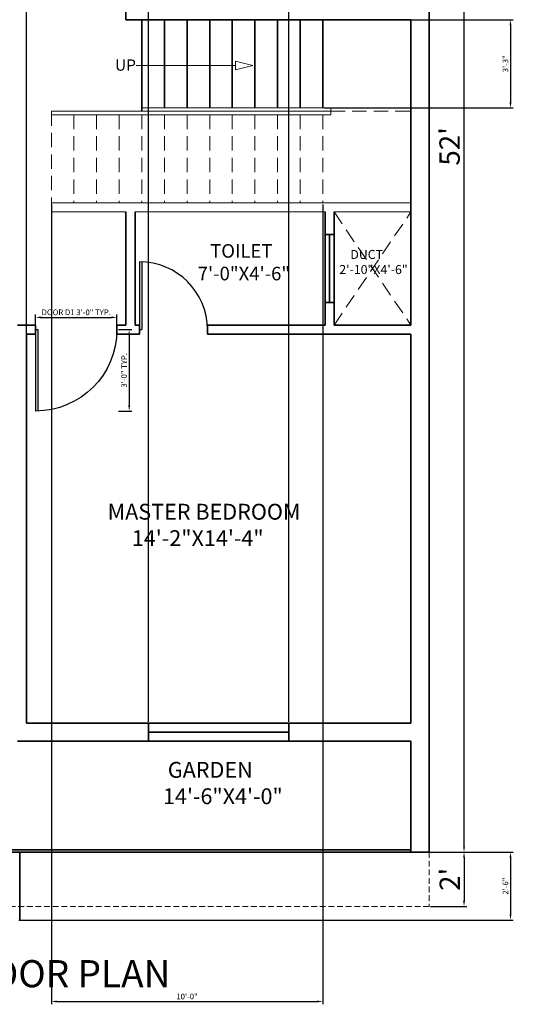
# Model space of a CAD drawing. Units: inches. Extents: x 1566 to 2546, y 1087 to 2705.
# Tile 25 of 27: x 1821 to 2039, y 1974 to 2409. Entities that reach past the tile are written whole.
import ezdxf

# ---------------------------------------------------------------- set-up
doc = ezdxf.new("R2010")
doc.units = ezdxf.units.IN
doc.linetypes.add('DASHED', pattern=[19.05, 12.7, -6.35])
for name, color, linetype, lineweight in [('A-ANNO-DIMS', 2, 'Continuous', 18), ('A-ANNO-TEXT', 7, 'Continuous', 18), ('A-AREA-IDEN', 7, 'Continuous', 18), ('A-DOOR', 4, 'Continuous', 25), ('A-FLOR-OVHD', 8, 'DASHED', 18), ('A-FLOR-STRS', 3, 'Continuous', 18), ('A-WALL', 7, 'Continuous', 35)]:
    doc.layers.add(name, color=color, linetype=linetype, lineweight=lineweight)
doc.styles.get("Standard").update_dxf_attribs({"font": 'arial.ttf'})
doc.dimstyles.new('ISO-25', dxfattribs={"dimtxt": 2.5, "dimasz": 2.5, "dimexe": 1.25, "dimexo": 0.625, "dimtad": 1, "dimtxsty": 'Standard', "dimcen": 2.5, "dimadec": 0, "dimazin": 0, "dimtfac": 1, "dimtmove": 0, "dimatfit": 3, "dimfxl": 1, "dimarcsym": 0})

# ---------------------------------------------------------------- blocks, each defined once
blk = doc.blocks.new('d2')
for p, q in [((3364.08, 1632.29), (3364.08, 1602.29)), ((3365.08, 1632.29), (3365.08, 1602.29)), ((3364.08, 1602.29), (3365.08, 1602.29))]:
    blk.add_line(p, q)
at = {"ltscale": 0.3}
blk.add_arc((3364.08, 1602.29), 30, 0, 90, dxfattribs=at)
blk = doc.blocks.new('d1')
for p, q in [((3297.32, 1596.93), (3297.32, 1632.93)), ((3298.32, 1596.93), (3298.32, 1632.93)), ((3297.32, 1596.93), (3298.32, 1596.93))]:
    blk.add_line(p, q)
at = {"ltscale": 0.3}
blk.add_arc((3297.32, 1596.93), 36, 0, 90, dxfattribs=at)
blk = doc.blocks.new('*D12')
at = {"layer": 'A-ANNO-DIMS', "color": 0, "lineweight": -2, "transparency": 16777216}
for p, q in [((2002.15, 2665.35), (2018.24, 2665.35)), ((2016.99, 2043.85), (2016.99, 2662.85)), ((2002.15, 2041.35), (2018.24, 2041.35))]:
    blk.add_line(p, q, dxfattribs=at)
at = {"layer": 'A-ANNO-DIMS', "color": 0, "transparency": 16777216}
for points in [[(2016.58, 2662.85), (2017.41, 2662.85), (2016.99, 2665.35)], [(2016.58, 2043.85), (2017.41, 2043.85), (2016.99, 2041.35)]]:
    blk.add_solid(points, dxfattribs=at)
at = {"layer": 'Defpoints', "color": 0, "transparency": 16777216}
for p in [(2001.53, 2665.35), (2016.99, 2665.35), (2001.53, 2041.35)]:
    blk.add_point(p, dxfattribs=at)
at = {"layer": 'A-ANNO-DIMS', "color": 0, "transparency": 16777216, "insert": (2011.77, 2353.35), "char_height": 9, "attachment_point": 5, "rotation": 90}
blk.add_mtext("52'", dxfattribs=at)
blk = doc.blocks.new('*D14')
at = {"layer": 'A-ANNO-DIMS', "color": 0, "lineweight": -2, "transparency": 16777216}
for p, q in [((2002.15, 2041.35), (2018.24, 2041.35)), ((2016.99, 2038.85), (2016.99, 2019.85)), ((2002.15, 2017.35), (2018.24, 2017.35))]:
    blk.add_line(p, q, dxfattribs=at)
at = {"layer": 'A-ANNO-DIMS', "color": 0, "transparency": 16777216}
for points in [[(2016.58, 2038.85), (2017.41, 2038.85), (2016.99, 2041.35)], [(2016.58, 2019.85), (2017.41, 2019.85), (2016.99, 2017.35)]]:
    blk.add_solid(points, dxfattribs=at)
at = {"layer": 'Defpoints', "color": 0, "transparency": 16777216}
for p in [(2001.53, 2041.35), (2001.53, 2017.35), (2016.99, 2017.35)]:
    blk.add_point(p, dxfattribs=at)
at = {"layer": 'A-ANNO-DIMS', "color": 0, "transparency": 16777216, "insert": (2011.85, 2029.35), "char_height": 9, "attachment_point": 5, "rotation": 90}
blk.add_mtext("2'", dxfattribs=at)
blk = doc.blocks.new('*D35')
at = {"layer": 'A-ANNO-DIMS', "color": 0, "lineweight": -2, "transparency": 16777216}
for p, q in [((1827.53, 2272.97), (1827.53, 2279)), ((1830.03, 2277.75), (1861.03, 2277.75)), ((1863.53, 2272.97), (1863.53, 2279))]:
    blk.add_line(p, q, dxfattribs=at)
at = {"layer": 'A-ANNO-DIMS', "color": 0, "transparency": 16777216}
for points in [[(1830.03, 2278.16), (1830.03, 2277.33), (1827.53, 2277.75)], [(1861.03, 2278.16), (1861.03, 2277.33), (1863.53, 2277.75)]]:
    blk.add_solid(points, dxfattribs=at)
at = {"layer": 'Defpoints', "color": 0, "transparency": 16777216}
for p in [(1863.53, 2277.75), (1827.53, 2272.35), (1863.53, 2272.35)]:
    blk.add_point(p, dxfattribs=at)
at = {"layer": 'A-ANNO-DIMS', "color": 0, "transparency": 16777216, "insert": (1845.53, 2279.67), "char_height": 2.5, "attachment_point": 5}
blk.add_mtext('DOOR D1 3\'-0" TYP.', dxfattribs=at)
blk = doc.blocks.new('*D36')
at = {"layer": 'A-ANNO-DIMS', "color": 0, "lineweight": -2, "transparency": 16777216}
for p, q in [((1864.15, 2272.35), (1870.18, 2272.35)), ((1868.93, 2269.85), (1868.93, 2238.85)), ((1864.15, 2236.35), (1870.18, 2236.35))]:
    blk.add_line(p, q, dxfattribs=at)
at = {"layer": 'A-ANNO-DIMS', "color": 0, "transparency": 16777216}
for points in [[(1868.51, 2269.85), (1869.35, 2269.85), (1868.93, 2272.35)], [(1868.51, 2238.85), (1869.35, 2238.85), (1868.93, 2236.35)]]:
    blk.add_solid(points, dxfattribs=at)
at = {"layer": 'Defpoints', "color": 0, "transparency": 16777216}
for p in [(1863.53, 2272.35), (1863.53, 2236.35), (1868.93, 2236.35)]:
    blk.add_point(p, dxfattribs=at)
at = {"layer": 'A-ANNO-DIMS', "color": 0, "transparency": 16777216, "insert": (1867.03, 2254.35), "char_height": 2.5, "attachment_point": 5, "rotation": 90}
blk.add_mtext('3\'-0" TYP.', dxfattribs=at)
blk = doc.blocks.new('*D81')
at = {"layer": 'A-ANNO-DIMS', "color": 0, "lineweight": -2, "transparency": 16777216}
for p, q in [((1823.53, 2098.97), (1823.53, 2702.6)), ((1826.03, 2701.35), (1875.03, 2701.35)), ((1877.53, 2098.97), (1877.53, 2702.6))]:
    blk.add_line(p, q, dxfattribs=at)
at = {"layer": 'A-ANNO-DIMS', "color": 0, "transparency": 16777216}
for points in [[(1826.03, 2701.76), (1826.03, 2700.93), (1823.53, 2701.35)], [(1875.03, 2701.76), (1875.03, 2700.93), (1877.53, 2701.35)]]:
    blk.add_solid(points, dxfattribs=at)
at = {"layer": 'Defpoints', "color": 0, "transparency": 16777216}
for p in [(1877.53, 2701.35), (1823.53, 2098.35), (1877.53, 2098.35)]:
    blk.add_point(p, dxfattribs=at)
at = {"layer": 'A-ANNO-DIMS', "color": 0, "transparency": 16777216, "insert": (1850.53, 2703.25), "char_height": 2.5, "attachment_point": 5}
blk.add_mtext('4\'-6"', dxfattribs=at)
blk = doc.blocks.new('*D82')
at = {"layer": 'A-ANNO-DIMS', "color": 0, "lineweight": -2, "transparency": 16777216}
for p, q in [((1877.53, 2098.97), (1877.53, 2702.6)), ((1880.03, 2701.35), (1937.03, 2701.35)), ((1939.53, 2098.97), (1939.53, 2702.6))]:
    blk.add_line(p, q, dxfattribs=at)
at = {"layer": 'A-ANNO-DIMS', "color": 0, "transparency": 16777216}
for points in [[(1880.03, 2701.76), (1880.03, 2700.93), (1877.53, 2701.35)], [(1937.03, 2701.76), (1937.03, 2700.93), (1939.53, 2701.35)]]:
    blk.add_solid(points, dxfattribs=at)
at = {"layer": 'Defpoints', "color": 0, "transparency": 16777216}
for p in [(1939.53, 2701.35), (1877.53, 2098.35), (1939.53, 2098.35)]:
    blk.add_point(p, dxfattribs=at)
at = {"layer": 'A-ANNO-DIMS', "color": 0, "transparency": 16777216, "insert": (1908.53, 2703.25), "char_height": 2.5, "attachment_point": 5}
blk.add_mtext('5\'-2"', dxfattribs=at)
blk = doc.blocks.new('*D84')
at = {"layer": 'A-ANNO-DIMS', "color": 0, "lineweight": -2, "transparency": 16777216}
for p, q in [((1955.15, 2409.35), (2038.78, 2409.35)), ((2037.53, 2406.85), (2037.53, 2372.85)), ((1955.15, 2370.35), (2038.78, 2370.35))]:
    blk.add_line(p, q, dxfattribs=at)
at = {"layer": 'A-ANNO-DIMS', "color": 0, "transparency": 16777216}
for points in [[(2037.11, 2406.85), (2037.95, 2406.85), (2037.53, 2409.35)], [(2037.11, 2372.85), (2037.95, 2372.85), (2037.53, 2370.35)]]:
    blk.add_solid(points, dxfattribs=at)
at = {"layer": 'Defpoints', "color": 0, "transparency": 16777216}
for p in [(1954.53, 2409.35), (1954.53, 2370.35), (2037.53, 2370.35)]:
    blk.add_point(p, dxfattribs=at)
at = {"layer": 'A-ANNO-DIMS', "color": 0, "transparency": 16777216, "insert": (2035.63, 2389.85), "char_height": 2.5, "attachment_point": 5, "rotation": 90}
blk.add_mtext('3\'-3"', dxfattribs=at)
blk = doc.blocks.new('*D85')
at = {"layer": 'A-ANNO-DIMS', "color": 0, "lineweight": -2, "transparency": 16777216}
for p, q in [((1834.53, 2327.72), (1834.53, 1974.1)), ((1954.53, 2327.72), (1954.53, 1974.1)), ((1837.03, 1975.35), (1952.03, 1975.35))]:
    blk.add_line(p, q, dxfattribs=at)
at = {"layer": 'A-ANNO-DIMS', "color": 0, "transparency": 16777216}
for points in [[(1837.03, 1975.76), (1837.03, 1974.93), (1834.53, 1975.35)], [(1952.03, 1975.76), (1952.03, 1974.93), (1954.53, 1975.35)]]:
    blk.add_solid(points, dxfattribs=at)
at = {"layer": 'Defpoints', "color": 0, "transparency": 16777216}
for p in [(1834.53, 2328.35), (1954.53, 2328.35), (1954.53, 1975.35)]:
    blk.add_point(p, dxfattribs=at)
at = {"layer": 'A-ANNO-DIMS', "color": 0, "transparency": 16777216, "insert": (1894.53, 1977.25), "char_height": 2.5, "attachment_point": 5}
blk.add_mtext('10\'-0"', dxfattribs=at)
blk = doc.blocks.new('*D87')
at = {"layer": 'A-ANNO-DIMS', "color": 0, "lineweight": -2, "transparency": 16777216}
for p, q in [((1821.15, 2041.35), (2038.78, 2041.35)), ((2037.53, 2038.85), (2037.53, 2013.85)), ((1820.15, 2011.35), (2038.78, 2011.35))]:
    blk.add_line(p, q, dxfattribs=at)
at = {"layer": 'A-ANNO-DIMS', "color": 0, "transparency": 16777216}
for points in [[(2037.11, 2038.85), (2037.95, 2038.85), (2037.53, 2041.35)], [(2037.11, 2013.85), (2037.95, 2013.85), (2037.53, 2011.35)]]:
    blk.add_solid(points, dxfattribs=at)
at = {"layer": 'Defpoints', "color": 0, "transparency": 16777216}
for p in [(1820.53, 2041.35), (1819.53, 2011.35), (2037.53, 2011.35)]:
    blk.add_point(p, dxfattribs=at)
at = {"layer": 'A-ANNO-DIMS', "color": 0, "transparency": 16777216, "insert": (2035.63, 2026.35), "char_height": 2.5, "attachment_point": 5, "rotation": 90}
blk.add_mtext('2\'-6"', dxfattribs=at)

msp = doc.modelspace()

# ---------------------------------------------------------------- linework, layer by layer
at = {"layer": 'A-FLOR-OVHD', "ltscale": 0.5}
for p, q in [((1834.53, 2368.85), (1834.53, 2324.35)), ((1958.03, 2368.85), (1993.53, 2368.85)), ((1844.53, 2367.35), (1844.53, 2328.35)), ((1854.53, 2367.35), (1854.53, 2328.35)), ((1864.53, 2367.35), (1864.53, 2328.35)), ((1874.53, 2367.35), (1874.53, 2328.35)), ((1884.53, 2367.35), (1884.53, 2328.35)), ((1894.53, 2367.35), (1894.53, 2328.35)), ((1904.53, 2367.35), (1904.53, 2328.35)), ((1914.53, 2367.35), (1914.53, 2328.35)), ((1924.53, 2367.35), (1924.53, 2328.35)), ((1934.53, 2367.35), (1934.53, 2328.35)), ((1944.53, 2367.35), (1944.53, 2328.35)), ((1954.53, 2367.35), (1954.53, 2328.35)), ((1959.53, 2324.35), (1993.53, 2274.35)), ((1959.53, 2274.35), (1993.53, 2324.35))]:
    msp.add_line(p, q, dxfattribs=at)
at = {"layer": 'A-FLOR-OVHD', "ltscale": 0.2}
for p, q in [((2001.53, 2041.35), (2001.53, 2017.35)), ((2001.53, 2017.35), (1605.53, 2017.35))]:
    msp.add_line(p, q, dxfattribs=at)
at = {"layer": 'A-FLOR-STRS'}
for p, q in [((1872.1, 2389.1), (1915.97, 2389.1)), ((1958.03, 2368.85), (1834.53, 2368.85)), ((1874.53, 2370.35), (1958.03, 2370.35)), ((1958.03, 2370.35), (1958.03, 2367.35)), ((1834.53, 2367.35), (1958.03, 2367.35)), ((1874.53, 2367.35), (1874.53, 2366.85)), ((1834.53, 2328.35), (1993.53, 2328.35)), ((1834.53, 2324.35), (1867.53, 2324.35)), ((1871.53, 2324.35), (1955.53, 2324.35)), ((1959.53, 2324.35), (1993.53, 2324.35))]:
    msp.add_line(p, q, dxfattribs=at)
msp.add_lwpolyline([(1923.62, 2389.1), (1915.97, 2390.95), (1915.97, 2387.24)], close=True, dxfattribs=at)
at = {"layer": 'A-WALL'}
for p, q in [((2001.53, 2665.35), (2001.53, 2041.35)), ((1867.53, 2493.35), (1867.53, 2409.35)), ((1867.53, 2409.35), (1993.53, 2409.35)), ((1874.53, 2409.35), (1874.53, 2368.85)), ((1884.53, 2409.35), (1884.53, 2370.35)), ((1894.53, 2409.35), (1894.53, 2370.35)), ((1904.53, 2409.35), (1904.53, 2370.35)), ((1914.53, 2409.35), (1914.53, 2370.35)), ((1924.53, 2409.35), (1924.53, 2370.35)), ((1934.53, 2409.35), (1934.53, 2370.35)), ((1944.53, 2409.35), (1944.53, 2370.35)), ((1954.53, 2409.35), (1954.53, 2370.35)), ((1993.53, 2409.35), (1993.53, 2274.35)), ((1867.53, 2324.35), (1867.53, 2274.35)), ((1871.53, 2324.35), (1871.53, 2274.35)), ((1955.53, 2324.35), (1955.53, 2274.35)), ((1959.53, 2324.35), (1959.53, 2274.35)), ((1955.53, 2314.35), (1959.53, 2314.35)), ((1957.53, 2314.35), (1957.53, 2284.35)), ((1955.53, 2284.35), (1959.53, 2284.35)), ((1819.53, 2274.35), (1827.53, 2274.35)), ((1827.53, 2270.35), (1827.53, 2274.35)), ((1863.53, 2274.35), (1867.53, 2274.35)), ((1863.53, 2270.35), (1863.53, 2274.35)), ((1871.53, 2274.35), (1873.53, 2274.35)), ((1873.53, 2274.35), (1873.53, 2270.35)), ((1903.53, 2274.35), (1955.53, 2274.35)), ((1903.53, 2274.35), (1903.53, 2270.35)), ((1959.53, 2274.35), (1993.53, 2274.35)), ((1823.53, 2270.35), (1827.53, 2270.35)), ((1823.53, 2098.35), (1823.53, 2270.35)), ((1863.53, 2270.35), (1873.53, 2270.35)), ((1903.53, 2270.35), (1993.53, 2270.35)), ((1993.53, 2270.35), (1993.53, 2098.35)), ((1823.53, 2098.35), (1993.53, 2098.35)), ((1877.53, 2098.35), (1877.53, 2090.35)), ((1877.53, 2098.35), (1877.53, 2090.35)), ((1939.53, 2098.35), (1939.53, 2090.35)), ((1939.53, 2098.35), (1939.53, 2090.35)), ((1877.53, 2094.35), (1939.53, 2094.35)), ((1877.53, 2094.35), (1939.53, 2094.35)), ((1819.53, 2090.35), (1993.53, 2090.35)), ((1993.53, 2090.35), (1993.53, 2041.35)), ((2001.53, 2041.35), (1641.53, 2041.35)), ((1993.53, 2042.35), (1745.53, 2042.35)), ((1820.53, 2041.35), (1820.53, 2011.35))]:
    msp.add_line(p, q, dxfattribs=at)

# ---------------------------------------------------------------- block references
at = {"layer": 'A-DOOR'}
msp.add_blockref('d2', (-1490.55, 670.05), dxfattribs=at)
at = {"layer": 'A-DOOR', "xscale": -1, "rotation": 180}
msp.add_blockref('d1', (-1469.79, 3869.27), dxfattribs=at)

# ---------------------------------------------------------------- texts
at = {"layer": 'A-ANNO-TEXT'}
msp.add_text('UP', height=5, dxfattribs=at).set_placement((1862.68, 2386.79))
at = {"layer": 'A-AREA-IDEN', "attachment_point": 1}
for s, width, insert, char_height in [('   TOILET\\P7\'-0"X4\'-6"', 111.7553, (1899.25, 2310.13), 6), ('    DUCT\\P2\'-10"X4\'-6"', 111.7553, (1961.83, 2307.57), 4), ('MASTER BEDROOM\\P     14\'-2"X14\'-4"', 111.7553, (1859.41, 2195.34), 7), (' GARDEN\\P14\'-6"X4\'-0"', 111.7553, (1883.88, 2081.24), 7), ('GROUND FLOOR PLAN', 267.5424, (1717.44, 1993.63), 12)]:
    msp.add_mtext_dynamic_manual_height_columns(s, width=width, gutter_width=12.5, heights=[0], dxfattribs=dict(at, insert=insert, char_height=char_height))

# ---------------------------------------------------------------- dimensions: what is measured, and where the dimension line sits
at = {"layer": 'A-ANNO-DIMS'}
for base, p1, p2, picture, middle in [((1877.53, 2701.35), (1823.53, 2098.35), (1877.53, 2098.35), '*D81', (1850.53, 2703.25)), ((1939.53, 2701.35), (1877.53, 2098.35), (1939.53, 2098.35), '*D82', (1908.53, 2703.25)), ((1954.53, 1975.35), (1834.53, 2328.35), (1954.53, 2328.35), '*D85', (1894.53, 1977.25))]:
    dim = msp.add_linear_dim(base=base, p1=p1, p2=p2, dimstyle='ISO-25', override={"dimdec": 1, "dimlfac": 1, "dimrnd": 0, "dimzin": 1, "dimdsep": 46, "dimlunit": 4, "dimfrac": 2}, dxfattribs=at)
    dim.commit()
    dim.dimension.update_dxf_attribs({"geometry": picture, "text_midpoint": middle})
for base, p1, p2, override, picture, middle in [((2016.99, 2665.35), (2001.53, 2041.35), (2001.53, 2665.35), {"dimtxt": 9, "dimdec": 1, "dimlunit": 3, "dimclrd": 0, "dimclre": 0, "dimclrt": 0, "dimtdec": 1}, '*D12', (2011.77, 2353.35)), ((2037.53, 2370.35), (1954.53, 2409.35), (1954.53, 2370.35), {"dimdec": 1, "dimlfac": 1, "dimrnd": 0, "dimzin": 1, "dimdsep": 46, "dimlunit": 4, "dimfrac": 2}, '*D84', (2035.63, 2389.85)), ((2037.53, 2011.35), (1820.53, 2041.35), (1819.53, 2011.35), {"dimdec": 1, "dimlfac": 1, "dimrnd": 0, "dimzin": 1, "dimdsep": 46, "dimlunit": 4, "dimfrac": 2}, '*D87', (2035.63, 2026.35)), ((2016.99, 2017.35), (2001.53, 2041.35), (2001.53, 2017.35), {"dimtxt": 9, "dimdec": 1, "dimlunit": 3, "dimclrd": 0, "dimclre": 0, "dimclrt": 0, "dimtdec": 1}, '*D14', (2011.85, 2029.35))]:
    dim = msp.add_linear_dim(base=base, p1=p1, p2=p2, angle=90, dimstyle='ISO-25', override=override, dxfattribs=at)
    dim.commit()
    dim.dimension.update_dxf_attribs({"geometry": picture, "text_midpoint": middle})
dim = msp.add_linear_dim(base=(1863.53, 2277.75), p1=(1827.53, 2272.35), p2=(1863.53, 2272.35), text='DOOR D1 <> TYP.', dimstyle='ISO-25', override={"dimdec": 1, "dimrnd": 0, "dimzin": 1, "dimlunit": 4, "dimfrac": 2}, dxfattribs=at)
dim.commit()
dim.dimension.update_dxf_attribs({"geometry": '*D35', "text_midpoint": (1845.53, 2279.67)})
dim = msp.add_linear_dim(base=(1868.93, 2236.35), p1=(1863.53, 2272.35), p2=(1863.53, 2236.35), angle=270, text='<> TYP.', dimstyle='ISO-25', override={"dimdec": 1, "dimrnd": 0, "dimzin": 1, "dimlunit": 4, "dimfrac": 2}, dxfattribs=at)
dim.commit()
dim.dimension.update_dxf_attribs({"geometry": '*D36', "text_midpoint": (1867.03, 2254.35)})

doc.saveas('drawing.dxf')
